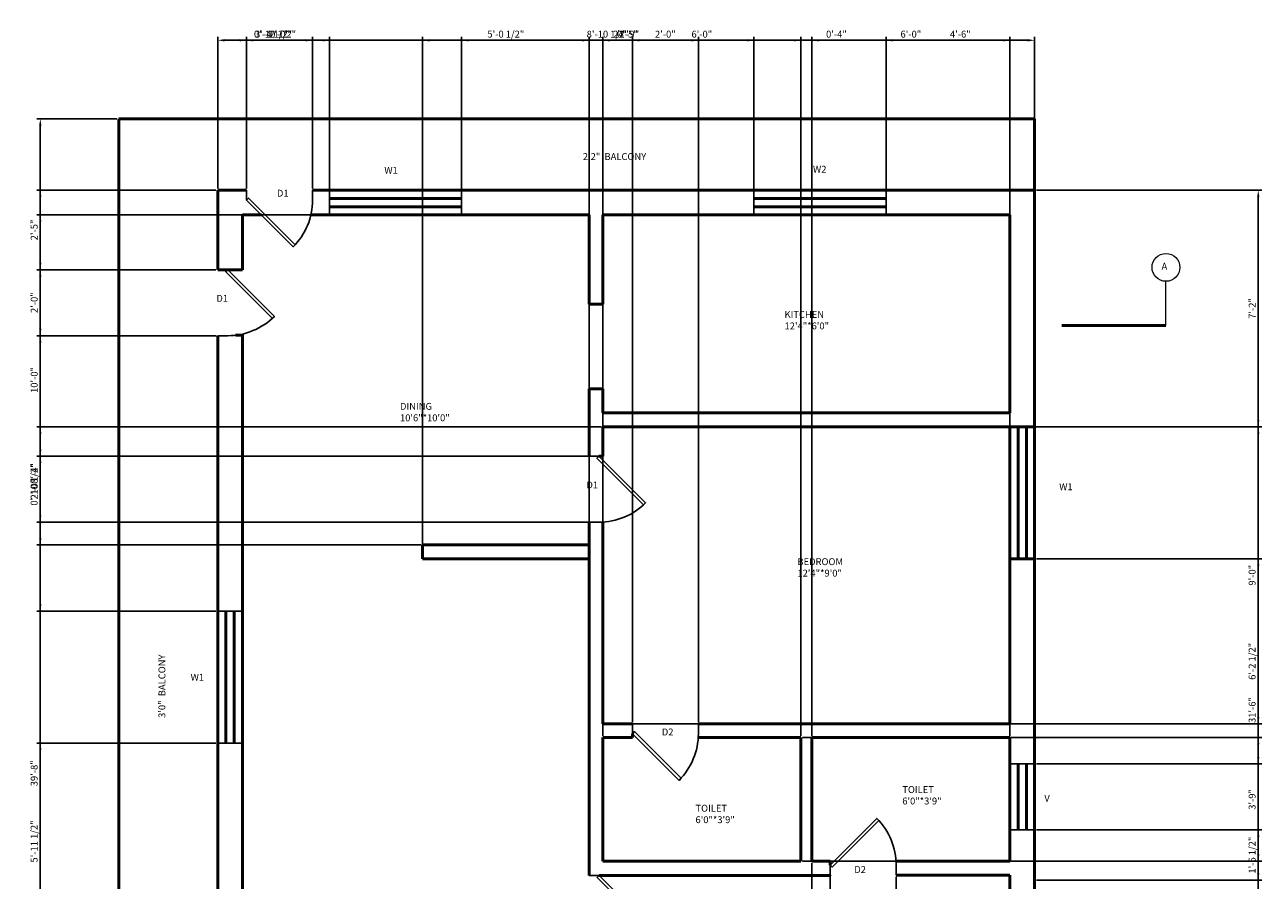
# Model space of a CAD drawing. Units: inches. Extents: x 2020 to 7901, y 1581 to 3943.
# Tile 11 of 17: x 2936 to 3386, y 1963 to 2274. Entities that reach past the tile are written whole.
import ezdxf

# ---------------------------------------------------------------- set-up
doc = ezdxf.new("R2010")
doc.units = ezdxf.units.IN
for name, color, linetype, lineweight in [('A-ANNO-DIMS', 2, 'Continuous', 18), ('A-ANNO-SYMB', 1, 'Continuous', 18), ('A-ANNO-TEXT', 7, 'Continuous', 18), ('A-AREA-IDEN', 3, 'Continuous', 18), ('A-DOOR', 4, 'Continuous', 25), ('A-GLAZ', 4, 'Continuous', 25), ('A-WALL', 7, 'Continuous', 50)]:
    doc.layers.add(name, color=color, linetype=linetype, lineweight=lineweight)
doc.styles.get("Standard").update_dxf_attribs({"font": 'arial.ttf'})
doc.dimstyles.new('ISO-25', dxfattribs={"dimtxt": 2.5, "dimasz": 2.5, "dimexe": 1.25, "dimexo": 0.625, "dimtad": 1, "dimdec": 1, "dimlunit": 3, "dimtxsty": 'Standard', "dimcen": 2.5, "dimadec": 0, "dimazin": 0, "dimtfac": 1, "dimtdec": 1, "dimtmove": 0, "dimatfit": 3, "dimfxl": 1, "dimarcsym": 0})

# ---------------------------------------------------------------- blocks, each defined once
blk = doc.blocks.new('*U10')
for p, q in [((0, 0), (0, -6)), ((40, 0), (40, -6))]:
    blk.add_line(p, q)
blk.add_lwpolyline([(0, 0), (28.28, 28.28), (29.52, 27.05), (1.24, -1.24)], close=True)
blk.add_arc((0, 0), 40, 0, 45)
blk = doc.blocks.new('WIN-1200')
for p, q in [((0, 9), (48, 9)), ((0, 0), (0, 9)), ((48, 9), (48, 0)), ((48, 0), (0, 0))]:
    blk.add_line(p, q)
blk = doc.blocks.new('VENT-600')
for p, q in [((0, 24), (9, 24)), ((0, 24), (0, 0)), ((9, 0), (9, 24)), ((0, 0), (9, 0))]:
    blk.add_line(p, q)
blk = doc.blocks.new('*D44')
at = {"layer": 'A-ANNO-DIMS', "color": 0, "lineweight": -2, "transparency": 16777216}
for p, q in [((3006.32, 2214.96), (3006.32, 2270.09)), ((3046.95, 2214.96), (3046.95, 2270.09)), ((3008.82, 2268.84), (3044.45, 2268.84))]:
    blk.add_line(p, q, dxfattribs=at)
at = {"layer": 'A-ANNO-DIMS', "color": 0, "transparency": 16777216}
for points in [[(3008.82, 2269.26), (3008.82, 2268.42), (3006.32, 2268.84)], [(3044.45, 2269.26), (3044.45, 2268.42), (3046.95, 2268.84)]]:
    blk.add_solid(points, dxfattribs=at)
at = {"layer": 'DEFPOINTS', "color": 0, "transparency": 16777216}
for p in [(3046.95, 2268.84), (3006.32, 2214.34), (3046.95, 2214.34)]:
    blk.add_point(p, dxfattribs=at)
at = {"layer": 'A-ANNO-DIMS', "color": 0, "transparency": 16777216, "insert": (3026.63, 2270.76), "char_height": 2.5, "attachment_point": 5}
blk.add_mtext('3\'-4 1/2"', dxfattribs=at)
blk = doc.blocks.new('*D45')
at = {"layer": 'A-ANNO-DIMS', "color": 0, "lineweight": -2, "transparency": 16777216}
for p, q in [((3094.95, 2214.96), (3094.95, 2270.09)), ((3201.28, 2214.96), (3201.28, 2270.09)), ((3097.45, 2268.84), (3198.78, 2268.84))]:
    blk.add_line(p, q, dxfattribs=at)
at = {"layer": 'A-ANNO-DIMS', "color": 0, "transparency": 16777216}
for points in [[(3097.45, 2269.26), (3097.45, 2268.42), (3094.95, 2268.84)], [(3198.78, 2269.26), (3198.78, 2268.42), (3201.28, 2268.84)]]:
    blk.add_solid(points, dxfattribs=at)
at = {"layer": 'DEFPOINTS', "color": 0, "transparency": 16777216}
for p in [(3201.28, 2268.84), (3094.95, 2214.34), (3201.28, 2214.34)]:
    blk.add_point(p, dxfattribs=at)
at = {"layer": 'A-ANNO-DIMS', "color": 0, "transparency": 16777216, "insert": (3148.11, 2270.76), "char_height": 2.5, "attachment_point": 5}
blk.add_mtext('8\'-10 1/2"', dxfattribs=at)
blk = doc.blocks.new('*D46')
at = {"layer": 'A-ANNO-DIMS', "color": 0, "lineweight": -2, "transparency": 16777216}
for p, q in [((3249.28, 2214.96), (3249.28, 2270.09)), ((3303.32, 2214.96), (3303.32, 2270.09)), ((3251.78, 2268.84), (3300.82, 2268.84))]:
    blk.add_line(p, q, dxfattribs=at)
at = {"layer": 'A-ANNO-DIMS', "color": 0, "transparency": 16777216}
for points in [[(3251.78, 2269.26), (3251.78, 2268.42), (3249.28, 2268.84)], [(3300.82, 2269.26), (3300.82, 2268.42), (3303.32, 2268.84)]]:
    blk.add_solid(points, dxfattribs=at)
at = {"layer": 'DEFPOINTS', "color": 0, "transparency": 16777216}
for p in [(3303.32, 2268.84), (3249.28, 2214.34), (3303.32, 2214.34)]:
    blk.add_point(p, dxfattribs=at)
at = {"layer": 'A-ANNO-DIMS', "color": 0, "transparency": 16777216, "insert": (3276.3, 2270.74), "char_height": 2.5, "attachment_point": 5}
blk.add_mtext('4\'-6"', dxfattribs=at)
blk = doc.blocks.new('*D47')
at = {"layer": 'A-ANNO-DIMS', "color": 0, "lineweight": -2, "transparency": 16777216}
for p, q in [((3303.94, 2214.34), (3385.87, 2214.34)), ((3384.62, 2211.84), (3384.62, 2130.84)), ((3303.94, 2128.34), (3385.87, 2128.34))]:
    blk.add_line(p, q, dxfattribs=at)
at = {"layer": 'A-ANNO-DIMS', "color": 0, "transparency": 16777216}
for points in [[(3384.2, 2211.84), (3385.03, 2211.84), (3384.62, 2214.34)], [(3384.2, 2130.84), (3385.03, 2130.84), (3384.62, 2128.34)]]:
    blk.add_solid(points, dxfattribs=at)
at = {"layer": 'DEFPOINTS', "color": 0, "transparency": 16777216}
for p in [(3303.32, 2214.34), (3303.32, 2128.34), (3384.62, 2128.34)]:
    blk.add_point(p, dxfattribs=at)
at = {"layer": 'A-ANNO-DIMS', "color": 0, "transparency": 16777216, "insert": (3382.74, 2171.34), "char_height": 2.5, "attachment_point": 5, "rotation": 90}
blk.add_mtext('7\'-2"', dxfattribs=at)
blk = doc.blocks.new('*D48')
at = {"layer": 'A-ANNO-DIMS', "color": 0, "lineweight": -2, "transparency": 16777216}
for p, q in [((3303.94, 2080.34), (3385.87, 2080.34)), ((3384.62, 2077.84), (3384.62, 2008.22)), ((3303.94, 2005.72), (3385.87, 2005.72))]:
    blk.add_line(p, q, dxfattribs=at)
at = {"layer": 'A-ANNO-DIMS', "color": 0, "transparency": 16777216}
for points in [[(3384.2, 2077.84), (3385.03, 2077.84), (3384.62, 2080.34)], [(3384.2, 2008.22), (3385.03, 2008.22), (3384.62, 2005.72)]]:
    blk.add_solid(points, dxfattribs=at)
at = {"layer": 'DEFPOINTS', "color": 0, "transparency": 16777216}
for p in [(3303.32, 2080.34), (3303.32, 2005.72), (3384.62, 2005.72)]:
    blk.add_point(p, dxfattribs=at)
at = {"layer": 'A-ANNO-DIMS', "color": 0, "transparency": 16777216, "insert": (3382.7, 2043.03), "char_height": 2.5, "attachment_point": 5, "rotation": 90}
blk.add_mtext('6\'-2 1/2"', dxfattribs=at)
blk = doc.blocks.new('*D49')
at = {"layer": 'A-ANNO-DIMS', "color": 0, "lineweight": -2, "transparency": 16777216}
for p, q in [((3303.94, 1981.72), (3385.87, 1981.72)), ((3384.62, 1979.22), (3384.62, 1965.95)), ((3303.94, 1963.45), (3385.87, 1963.45))]:
    blk.add_line(p, q, dxfattribs=at)
at = {"layer": 'A-ANNO-DIMS', "color": 0, "transparency": 16777216}
for points in [[(3384.2, 1979.22), (3385.03, 1979.22), (3384.62, 1981.72)], [(3384.2, 1965.95), (3385.03, 1965.95), (3384.62, 1963.45)]]:
    blk.add_solid(points, dxfattribs=at)
at = {"layer": 'DEFPOINTS', "color": 0, "transparency": 16777216}
for p in [(3303.32, 1981.72), (3303.32, 1963.45), (3384.62, 1963.45)]:
    blk.add_point(p, dxfattribs=at)
at = {"layer": 'A-ANNO-DIMS', "color": 0, "transparency": 16777216, "insert": (3382.7, 1972.58), "char_height": 2.5, "attachment_point": 5, "rotation": 90}
blk.add_mtext('1\'-6 1/2"', dxfattribs=at)
blk = doc.blocks.new('*D55')
at = {"layer": 'A-ANNO-DIMS', "color": 0, "lineweight": -2, "transparency": 16777216}
for p, q in [((2969.69, 2240.34), (2940.57, 2240.34)), ((2941.82, 2237.84), (2941.82, 1766.84)), ((2969.69, 1764.34), (2940.57, 1764.34))]:
    blk.add_line(p, q, dxfattribs=at)
at = {"layer": 'A-ANNO-DIMS', "color": 0, "transparency": 16777216}
for points in [[(2941.4, 2237.84), (2942.23, 2237.84), (2941.82, 2240.34)], [(2941.4, 1766.84), (2942.23, 1766.84), (2941.82, 1764.34)]]:
    blk.add_solid(points, dxfattribs=at)
at = {"layer": 'DEFPOINTS', "color": 0, "transparency": 16777216}
for p in [(2970.32, 2240.34), (2941.82, 1764.34), (2970.32, 1764.34)]:
    blk.add_point(p, dxfattribs=at)
at = {"layer": 'A-ANNO-DIMS', "color": 0, "transparency": 16777216, "insert": (2939.91, 2002.34), "char_height": 2.5, "attachment_point": 5, "rotation": 90}
blk.add_mtext('39\'-8"', dxfattribs=at)
blk = doc.blocks.new('*D58')
at = {"layer": 'A-ANNO-DIMS', "color": 0, "lineweight": -2, "transparency": 16777216}
for p, q in [((3141.33, 2094.26), (3141.33, 2270.09)), ((3146.32, 2094.3), (3146.32, 2270.09)), ((3138.83, 2268.84), (3136.33, 2268.84)), ((3141.33, 2268.84), (3146.32, 2268.84)), ((3148.82, 2268.84), (3159.21, 2268.84))]:
    blk.add_line(p, q, dxfattribs=at)
at = {"layer": 'A-ANNO-DIMS', "color": 0, "transparency": 16777216}
for points in [[(3138.83, 2269.26), (3138.83, 2268.42), (3141.33, 2268.84)], [(3148.82, 2269.26), (3148.82, 2268.42), (3146.32, 2268.84)]]:
    blk.add_solid(points, dxfattribs=at)
at = {"layer": 'DEFPOINTS', "color": 0, "transparency": 16777216}
for p in [(3146.32, 2268.84), (3141.33, 2093.64), (3146.32, 2093.68)]:
    blk.add_point(p, dxfattribs=at)
at = {"layer": 'A-ANNO-DIMS', "color": 0, "transparency": 16777216, "insert": (3155.26, 2270.74), "char_height": 2.5, "attachment_point": 5}
blk.add_mtext('0\'-5"', dxfattribs=at)
blk = doc.blocks.new('*D59')
at = {"layer": 'A-ANNO-DIMS', "color": 0, "lineweight": -2, "transparency": 16777216}
for p, q in [((3157.06, 2020.96), (3157.06, 2270.09)), ((3181.06, 2020.96), (3181.06, 2270.09)), ((3159.56, 2268.84), (3178.56, 2268.84))]:
    blk.add_line(p, q, dxfattribs=at)
at = {"layer": 'A-ANNO-DIMS', "color": 0, "transparency": 16777216}
for points in [[(3159.56, 2269.26), (3159.56, 2268.42), (3157.06, 2268.84)], [(3178.56, 2269.26), (3178.56, 2268.42), (3181.06, 2268.84)]]:
    blk.add_solid(points, dxfattribs=at)
at = {"layer": 'DEFPOINTS', "color": 0, "transparency": 16777216}
for p in [(3181.06, 2268.84), (3157.06, 2020.34), (3181.06, 2020.34)]:
    blk.add_point(p, dxfattribs=at)
at = {"layer": 'A-ANNO-DIMS', "color": 0, "transparency": 16777216, "insert": (3169.06, 2270.74), "char_height": 2.5, "attachment_point": 5}
blk.add_mtext('2\'-0"', dxfattribs=at)
blk = doc.blocks.new('*D122')
at = {"layer": 'A-ANNO-DIMS', "color": 0, "lineweight": -2, "transparency": 16777216}
for p, q in [((3006.32, 2214.96), (3006.32, 2270.09)), ((3303.32, 2214.96), (3303.32, 2270.09)), ((3008.82, 2268.84), (3300.82, 2268.84))]:
    blk.add_line(p, q, dxfattribs=at)
at = {"layer": 'A-ANNO-DIMS', "color": 0, "transparency": 16777216}
for points in [[(3008.82, 2269.26), (3008.82, 2268.42), (3006.32, 2268.84)], [(3300.82, 2269.26), (3300.82, 2268.42), (3303.32, 2268.84)]]:
    blk.add_solid(points, dxfattribs=at)
at = {"layer": 'DEFPOINTS', "color": 0, "transparency": 16777216}
for p in [(3303.32, 2268.84), (3006.32, 2214.34), (3303.32, 2214.34)]:
    blk.add_point(p, dxfattribs=at)
at = {"layer": 'A-ANNO-DIMS', "color": 0, "transparency": 16777216, "insert": (3154.82, 2270.74), "char_height": 2.5, "attachment_point": 5}
blk.add_mtext('24\'-9"', dxfattribs=at)
blk = doc.blocks.new('*D123')
at = {"layer": 'A-ANNO-DIMS', "color": 0, "lineweight": -2, "transparency": 16777216}
for p, q in [((3303.94, 2214.34), (3385.87, 2214.34)), ((3384.62, 2211.84), (3384.62, 1838.84)), ((3303.94, 1836.34), (3385.87, 1836.34))]:
    blk.add_line(p, q, dxfattribs=at)
at = {"layer": 'A-ANNO-DIMS', "color": 0, "transparency": 16777216}
for points in [[(3384.2, 2211.84), (3385.03, 2211.84), (3384.62, 2214.34)], [(3384.2, 1838.84), (3385.03, 1838.84), (3384.62, 1836.34)]]:
    blk.add_solid(points, dxfattribs=at)
at = {"layer": 'DEFPOINTS', "color": 0, "transparency": 16777216}
for p in [(3303.32, 2214.34), (3303.32, 1836.34), (3384.62, 1836.34)]:
    blk.add_point(p, dxfattribs=at)
at = {"layer": 'A-ANNO-DIMS', "color": 0, "transparency": 16777216, "insert": (3382.71, 2025.34), "char_height": 2.5, "attachment_point": 5, "rotation": 90}
blk.add_mtext('31\'-6"', dxfattribs=at)
blk = doc.blocks.new('*D124')
at = {"layer": 'A-ANNO-DIMS', "color": 0, "lineweight": -2, "transparency": 16777216}
for p, q in [((3006.32, 2214.96), (3006.32, 2270.09)), ((3016.81, 2214.96), (3016.81, 2270.09)), ((3008.82, 2268.84), (3014.31, 2268.84)), ((3016.81, 2268.84), (3034.97, 2268.84))]:
    blk.add_line(p, q, dxfattribs=at)
at = {"layer": 'A-ANNO-DIMS', "color": 0, "transparency": 16777216}
for points in [[(3008.82, 2269.26), (3008.82, 2268.42), (3006.32, 2268.84)], [(3014.31, 2269.26), (3014.31, 2268.42), (3016.81, 2268.84)]]:
    blk.add_solid(points, dxfattribs=at)
at = {"layer": 'DEFPOINTS', "color": 0, "transparency": 16777216}
for p in [(3016.81, 2268.84), (3006.32, 2214.34), (3016.81, 2214.34)]:
    blk.add_point(p, dxfattribs=at)
at = {"layer": 'A-ANNO-DIMS', "color": 0, "transparency": 16777216, "insert": (3027.14, 2270.76), "char_height": 2.5, "attachment_point": 5}
blk.add_mtext('0\'-10 1/2"', dxfattribs=at)
blk = doc.blocks.new('*D125')
at = {"layer": 'A-ANNO-DIMS', "color": 0, "lineweight": -2, "transparency": 16777216}
for p, q in [((3016.81, 2214.96), (3016.81, 2270.09)), ((3040.81, 2214.96), (3040.81, 2270.09)), ((3019.31, 2268.84), (3038.31, 2268.84))]:
    blk.add_line(p, q, dxfattribs=at)
at = {"layer": 'A-ANNO-DIMS', "color": 0, "transparency": 16777216}
for points in [[(3019.31, 2269.26), (3019.31, 2268.42), (3016.81, 2268.84)], [(3038.31, 2269.26), (3038.31, 2268.42), (3040.81, 2268.84)]]:
    blk.add_solid(points, dxfattribs=at)
at = {"layer": 'DEFPOINTS', "color": 0, "transparency": 16777216}
for p in [(3040.81, 2268.84), (3016.81, 2214.34), (3040.81, 2214.34)]:
    blk.add_point(p, dxfattribs=at)
at = {"layer": 'A-ANNO-DIMS', "color": 0, "transparency": 16777216, "insert": (3028.81, 2270.74), "char_height": 2.5, "attachment_point": 5}
blk.add_mtext('2\'-0"', dxfattribs=at)
blk = doc.blocks.new('*D126')
at = {"layer": 'A-ANNO-DIMS', "color": 0, "lineweight": -2, "transparency": 16777216}
for p, q in [((3146.94, 2128.34), (3385.87, 2128.34)), ((3384.62, 2125.84), (3384.62, 2022.84)), ((3146.94, 2020.34), (3385.87, 2020.34))]:
    blk.add_line(p, q, dxfattribs=at)
at = {"layer": 'A-ANNO-DIMS', "color": 0, "transparency": 16777216}
for points in [[(3384.2, 2125.84), (3385.03, 2125.84), (3384.62, 2128.34)], [(3384.2, 2022.84), (3385.03, 2022.84), (3384.62, 2020.34)]]:
    blk.add_solid(points, dxfattribs=at)
at = {"layer": 'DEFPOINTS', "color": 0, "transparency": 16777216}
for p in [(3146.32, 2128.34), (3146.32, 2020.34), (3384.62, 2020.34)]:
    blk.add_point(p, dxfattribs=at)
at = {"layer": 'A-ANNO-DIMS', "color": 0, "transparency": 16777216, "insert": (3382.71, 2074.34), "char_height": 2.5, "attachment_point": 5, "rotation": 90}
blk.add_mtext('9\'-0"', dxfattribs=at)
blk = doc.blocks.new('*D127')
at = {"layer": 'A-ANNO-DIMS', "color": 0, "lineweight": -2, "transparency": 16777216}
for p, q in [((3218.94, 2015.34), (3385.87, 2015.34)), ((3384.62, 2012.84), (3384.62, 1972.84)), ((3218.94, 1970.34), (3385.87, 1970.34))]:
    blk.add_line(p, q, dxfattribs=at)
at = {"layer": 'A-ANNO-DIMS', "color": 0, "transparency": 16777216}
for points in [[(3384.2, 2012.84), (3385.03, 2012.84), (3384.62, 2015.34)], [(3384.2, 1972.84), (3385.03, 1972.84), (3384.62, 1970.34)]]:
    blk.add_solid(points, dxfattribs=at)
at = {"layer": 'DEFPOINTS', "color": 0, "transparency": 16777216}
for p in [(3218.32, 2015.34), (3218.32, 1970.34), (3384.62, 1970.34)]:
    blk.add_point(p, dxfattribs=at)
at = {"layer": 'A-ANNO-DIMS', "color": 0, "transparency": 16777216, "insert": (3382.71, 1992.84), "char_height": 2.5, "attachment_point": 5, "rotation": 90}
blk.add_mtext('3\'-9"', dxfattribs=at)
blk = doc.blocks.new('*D129')
at = {"layer": 'A-ANNO-DIMS', "color": 0, "lineweight": -2, "transparency": 16777216}
for p, q in [((3146.32, 2015.96), (3146.32, 2270.09)), ((3218.32, 2015.96), (3218.32, 2270.09)), ((3148.82, 2268.84), (3215.82, 2268.84))]:
    blk.add_line(p, q, dxfattribs=at)
at = {"layer": 'A-ANNO-DIMS', "color": 0, "transparency": 16777216}
for points in [[(3148.82, 2269.26), (3148.82, 2268.42), (3146.32, 2268.84)], [(3215.82, 2269.26), (3215.82, 2268.42), (3218.32, 2268.84)]]:
    blk.add_solid(points, dxfattribs=at)
at = {"layer": 'DEFPOINTS', "color": 0, "transparency": 16777216}
for p in [(3218.32, 2268.84), (3146.32, 2015.34), (3218.32, 2015.34)]:
    blk.add_point(p, dxfattribs=at)
at = {"layer": 'A-ANNO-DIMS', "color": 0, "transparency": 16777216, "insert": (3182.32, 2270.74), "char_height": 2.5, "attachment_point": 5}
blk.add_mtext('6\'-0"', dxfattribs=at)
blk = doc.blocks.new('*D130')
at = {"layer": 'A-ANNO-DIMS', "color": 0, "lineweight": -2, "transparency": 16777216}
for p, q in [((3218.32, 2015.96), (3218.32, 2270.09)), ((3222.32, 2015.96), (3222.32, 2270.09)), ((3215.82, 2268.84), (3213.32, 2268.84)), ((3218.32, 2268.84), (3222.32, 2268.84)), ((3224.82, 2268.84), (3235.21, 2268.84))]:
    blk.add_line(p, q, dxfattribs=at)
at = {"layer": 'A-ANNO-DIMS', "color": 0, "transparency": 16777216}
for points in [[(3215.82, 2269.26), (3215.82, 2268.42), (3218.32, 2268.84)], [(3224.82, 2269.26), (3224.82, 2268.42), (3222.32, 2268.84)]]:
    blk.add_solid(points, dxfattribs=at)
at = {"layer": 'DEFPOINTS', "color": 0, "transparency": 16777216}
for p in [(3222.32, 2268.84), (3218.32, 2015.34), (3222.32, 2015.34)]:
    blk.add_point(p, dxfattribs=at)
at = {"layer": 'A-ANNO-DIMS', "color": 0, "transparency": 16777216, "insert": (3231.26, 2270.74), "char_height": 2.5, "attachment_point": 5}
blk.add_mtext('0\'-4"', dxfattribs=at)
blk = doc.blocks.new('*D131')
at = {"layer": 'A-ANNO-DIMS', "color": 0, "lineweight": -2, "transparency": 16777216}
for p, q in [((3222.32, 2015.96), (3222.32, 2270.09)), ((3294.32, 2015.96), (3294.32, 2270.09)), ((3224.82, 2268.84), (3291.82, 2268.84))]:
    blk.add_line(p, q, dxfattribs=at)
at = {"layer": 'A-ANNO-DIMS', "color": 0, "transparency": 16777216}
for points in [[(3224.82, 2269.26), (3224.82, 2268.42), (3222.32, 2268.84)], [(3291.82, 2269.26), (3291.82, 2268.42), (3294.32, 2268.84)]]:
    blk.add_solid(points, dxfattribs=at)
at = {"layer": 'DEFPOINTS', "color": 0, "transparency": 16777216}
for p in [(3294.32, 2268.84), (3222.32, 2015.34), (3294.32, 2015.34)]:
    blk.add_point(p, dxfattribs=at)
at = {"layer": 'A-ANNO-DIMS', "color": 0, "transparency": 16777216, "insert": (3258.32, 2270.74), "char_height": 2.5, "attachment_point": 5}
blk.add_mtext('6\'-0"', dxfattribs=at)
blk = doc.blocks.new('*D132')
at = {"layer": 'A-ANNO-DIMS', "color": 0, "lineweight": -2, "transparency": 16777216}
for p, q in [((3094.33, 2205.34), (2940.57, 2205.34)), ((2941.82, 2202.84), (2941.82, 2087.84)), ((3080.19, 2085.34), (2940.57, 2085.34))]:
    blk.add_line(p, q, dxfattribs=at)
at = {"layer": 'A-ANNO-DIMS', "color": 0, "transparency": 16777216}
for points in [[(2941.4, 2202.84), (2942.23, 2202.84), (2941.82, 2205.34)], [(2941.4, 2087.84), (2942.23, 2087.84), (2941.82, 2085.34)]]:
    blk.add_solid(points, dxfattribs=at)
at = {"layer": 'DEFPOINTS', "color": 0, "transparency": 16777216}
for p in [(3094.95, 2205.34), (2941.82, 2085.34), (3080.82, 2085.34)]:
    blk.add_point(p, dxfattribs=at)
at = {"layer": 'A-ANNO-DIMS', "color": 0, "transparency": 16777216, "insert": (2939.92, 2145.34), "char_height": 2.5, "attachment_point": 5, "rotation": 90}
blk.add_mtext('10\'-0"', dxfattribs=at)
blk = doc.blocks.new('*D133')
at = {"layer": 'A-ANNO-DIMS', "color": 0, "lineweight": -2, "transparency": 16777216}
for p, q in [((3080.82, 2080.96), (3080.82, 2270.09)), ((3141.32, 2080.96), (3141.32, 2270.09)), ((3083.32, 2268.84), (3138.82, 2268.84))]:
    blk.add_line(p, q, dxfattribs=at)
at = {"layer": 'A-ANNO-DIMS', "color": 0, "transparency": 16777216}
for points in [[(3083.32, 2269.26), (3083.32, 2268.42), (3080.82, 2268.84)], [(3138.82, 2269.26), (3138.82, 2268.42), (3141.32, 2268.84)]]:
    blk.add_solid(points, dxfattribs=at)
at = {"layer": 'DEFPOINTS', "color": 0, "transparency": 16777216}
for p in [(3141.32, 2268.84), (3080.82, 2080.34), (3141.32, 2080.34)]:
    blk.add_point(p, dxfattribs=at)
at = {"layer": 'A-ANNO-DIMS', "color": 0, "transparency": 16777216, "insert": (3111.07, 2270.76), "char_height": 2.5, "attachment_point": 5}
blk.add_mtext('5\'-0 1/2"', dxfattribs=at)
blk = doc.blocks.new('*D134')
at = {"layer": 'A-ANNO-DIMS', "color": 0, "lineweight": -2, "transparency": 16777216}
for p, q in [((3145.69, 2128.34), (2940.57, 2128.34)), ((2941.82, 2125.84), (2941.82, 2120.14)), ((3145.69, 2117.64), (2940.57, 2117.64)), ((2941.82, 2117.64), (2941.82, 2099.47))]:
    blk.add_line(p, q, dxfattribs=at)
at = {"layer": 'A-ANNO-DIMS', "color": 0, "transparency": 16777216}
for points in [[(2941.4, 2125.84), (2942.23, 2125.84), (2941.82, 2128.34)], [(2941.4, 2120.14), (2942.23, 2120.14), (2941.82, 2117.64)]]:
    blk.add_solid(points, dxfattribs=at)
at = {"layer": 'DEFPOINTS', "color": 0, "transparency": 16777216}
for p in [(3146.32, 2128.34), (2941.82, 2117.64), (3146.32, 2117.64)]:
    blk.add_point(p, dxfattribs=at)
at = {"layer": 'A-ANNO-DIMS', "color": 0, "transparency": 16777216, "insert": (2939.9, 2107.31), "char_height": 2.5, "attachment_point": 5, "rotation": 90}
blk.add_mtext('0\'-10 1/2"', dxfattribs=at)
blk = doc.blocks.new('*D135')
at = {"layer": 'A-ANNO-DIMS', "color": 0, "lineweight": -2, "transparency": 16777216}
for p, q in [((3145.69, 2117.64), (2940.57, 2117.64)), ((2941.82, 2115.14), (2941.82, 2096.18)), ((3145.69, 2093.68), (2940.57, 2093.68))]:
    blk.add_line(p, q, dxfattribs=at)
at = {"layer": 'A-ANNO-DIMS', "color": 0, "transparency": 16777216}
for points in [[(2941.4, 2115.14), (2942.23, 2115.14), (2941.82, 2117.64)], [(2941.4, 2096.18), (2942.23, 2096.18), (2941.82, 2093.68)]]:
    blk.add_solid(points, dxfattribs=at)
at = {"layer": 'DEFPOINTS', "color": 0, "transparency": 16777216}
for p in [(3146.32, 2117.64), (2941.82, 2093.68), (3146.32, 2093.68)]:
    blk.add_point(p, dxfattribs=at)
at = {"layer": 'A-ANNO-DIMS', "color": 0, "transparency": 16777216, "insert": (2939.92, 2105.66), "char_height": 2.5, "attachment_point": 5, "rotation": 90}
blk.add_mtext('2\'-0"', dxfattribs=at)
blk = doc.blocks.new('*D136')
at = {"layer": 'A-ANNO-DIMS', "color": 0, "lineweight": -2, "transparency": 16777216}
for p, q in [((3222.32, 1969.71), (3222.32, 1734.59)), ((3228.97, 1969.71), (3228.97, 1734.59)), ((3224.82, 1735.84), (3226.47, 1735.84)), ((3228.97, 1735.84), (3245.19, 1735.84))]:
    blk.add_line(p, q, dxfattribs=at)
at = {"layer": 'A-ANNO-DIMS', "color": 0, "transparency": 16777216}
for points in [[(3224.82, 1736.26), (3224.82, 1735.42), (3222.32, 1735.84)], [(3226.47, 1736.26), (3226.47, 1735.42), (3228.97, 1735.84)]]:
    blk.add_solid(points, dxfattribs=at)
at = {"layer": 'DEFPOINTS', "color": 0, "transparency": 16777216}
for p in [(3222.32, 1970.34), (3228.97, 1970.34), (3228.97, 1735.84)]:
    blk.add_point(p, dxfattribs=at)
at = {"layer": 'A-ANNO-DIMS', "color": 0, "transparency": 16777216, "insert": (3238.33, 1737.76), "char_height": 2.5, "attachment_point": 5}
blk.add_mtext('0\'-6 1/2"', dxfattribs=at)
blk = doc.blocks.new('*D137')
at = {"layer": 'A-ANNO-DIMS', "color": 0, "lineweight": -2, "transparency": 16777216}
for p, q in [((3228.97, 1964.72), (3228.97, 1734.59)), ((3252.97, 1964.72), (3252.97, 1734.59)), ((3231.47, 1735.84), (3250.47, 1735.84))]:
    blk.add_line(p, q, dxfattribs=at)
at = {"layer": 'A-ANNO-DIMS', "color": 0, "transparency": 16777216}
for points in [[(3231.47, 1736.26), (3231.47, 1735.42), (3228.97, 1735.84)], [(3250.47, 1736.26), (3250.47, 1735.42), (3252.97, 1735.84)]]:
    blk.add_solid(points, dxfattribs=at)
at = {"layer": 'DEFPOINTS', "color": 0, "transparency": 16777216}
for p in [(3228.97, 1965.35), (3252.97, 1965.35), (3252.97, 1735.84)]:
    blk.add_point(p, dxfattribs=at)
at = {"layer": 'A-ANNO-DIMS', "color": 0, "transparency": 16777216, "insert": (3240.97, 1737.74), "char_height": 2.5, "attachment_point": 5}
blk.add_mtext('2\'-0"', dxfattribs=at)
blk = doc.blocks.new('*D140')
at = {"layer": 'A-ANNO-DIMS', "color": 0, "lineweight": -2, "transparency": 16777216}
for p, q in [((3005.69, 2214.34), (2940.57, 2214.34)), ((2941.82, 2211.84), (2941.82, 2187.94)), ((3005.69, 2185.44), (2940.57, 2185.44))]:
    blk.add_line(p, q, dxfattribs=at)
at = {"layer": 'A-ANNO-DIMS', "color": 0, "transparency": 16777216}
for points in [[(2941.4, 2211.84), (2942.23, 2211.84), (2941.82, 2214.34)], [(2941.4, 2187.94), (2942.23, 2187.94), (2941.82, 2185.44)]]:
    blk.add_solid(points, dxfattribs=at)
at = {"layer": 'DEFPOINTS', "color": 0, "transparency": 16777216}
for p in [(3006.32, 2214.34), (2941.82, 2185.44), (3006.32, 2185.44)]:
    blk.add_point(p, dxfattribs=at)
at = {"layer": 'A-ANNO-DIMS', "color": 0, "transparency": 16777216, "insert": (2939.92, 2199.89), "char_height": 2.5, "attachment_point": 5, "rotation": 90}
blk.add_mtext('2\'-5"', dxfattribs=at)
blk = doc.blocks.new('*D141')
at = {"layer": 'A-ANNO-DIMS', "color": 0, "lineweight": -2, "transparency": 16777216}
for p, q in [((3005.69, 2185.44), (2940.57, 2185.44)), ((2941.82, 2182.94), (2941.82, 2163.94)), ((3005.73, 2161.44), (2940.57, 2161.44))]:
    blk.add_line(p, q, dxfattribs=at)
at = {"layer": 'A-ANNO-DIMS', "color": 0, "transparency": 16777216}
for points in [[(2941.4, 2182.94), (2942.23, 2182.94), (2941.82, 2185.44)], [(2941.4, 2163.94), (2942.23, 2163.94), (2941.82, 2161.44)]]:
    blk.add_solid(points, dxfattribs=at)
at = {"layer": 'DEFPOINTS', "color": 0, "transparency": 16777216}
for p in [(3006.32, 2185.44), (2941.82, 2161.44), (3006.36, 2161.44)]:
    blk.add_point(p, dxfattribs=at)
at = {"layer": 'A-ANNO-DIMS', "color": 0, "transparency": 16777216, "insert": (2939.92, 2173.44), "char_height": 2.5, "attachment_point": 5, "rotation": 90}
blk.add_mtext('2\'-0"', dxfattribs=at)
blk = doc.blocks.new('*D142')
at = {"layer": 'A-ANNO-DIMS', "color": 0, "lineweight": -2, "transparency": 16777216}
for p, q in [((3005.73, 2161.44), (2940.57, 2161.44)), ((2941.82, 2158.94), (2941.82, 2063.8)), ((3005.69, 2061.3), (2940.57, 2061.3))]:
    blk.add_line(p, q, dxfattribs=at)
at = {"layer": 'A-ANNO-DIMS', "color": 0, "transparency": 16777216}
for points in [[(2941.4, 2158.94), (2942.23, 2158.94), (2941.82, 2161.44)], [(2941.4, 2063.8), (2942.23, 2063.8), (2941.82, 2061.3)]]:
    blk.add_solid(points, dxfattribs=at)
at = {"layer": 'DEFPOINTS', "color": 0, "transparency": 16777216}
for p in [(3006.36, 2161.44), (2941.82, 2061.3), (3006.32, 2061.3)]:
    blk.add_point(p, dxfattribs=at)
at = {"layer": 'A-ANNO-DIMS', "color": 0, "transparency": 16777216, "insert": (2939.92, 2111.37), "char_height": 2.5, "attachment_point": 5, "rotation": 90}
blk.add_mtext('8\'-4"', dxfattribs=at)
blk = doc.blocks.new('*D143')
at = {"layer": 'A-ANNO-DIMS', "color": 0, "lineweight": -2, "transparency": 16777216}
for p, q in [((3005.69, 2013.3), (2940.57, 2013.3)), ((2941.82, 2010.8), (2941.82, 1944.29)), ((3005.69, 1941.79), (2940.57, 1941.79))]:
    blk.add_line(p, q, dxfattribs=at)
at = {"layer": 'A-ANNO-DIMS', "color": 0, "transparency": 16777216}
for points in [[(2941.4, 2010.8), (2942.23, 2010.8), (2941.82, 2013.3)], [(2941.4, 1944.29), (2942.23, 1944.29), (2941.82, 1941.79)]]:
    blk.add_solid(points, dxfattribs=at)
at = {"layer": 'DEFPOINTS', "color": 0, "transparency": 16777216}
for p in [(3006.32, 2013.3), (2941.82, 1941.79), (3006.32, 1941.79)]:
    blk.add_point(p, dxfattribs=at)
at = {"layer": 'A-ANNO-DIMS', "color": 0, "transparency": 16777216, "insert": (2939.9, 1977.54), "char_height": 2.5, "attachment_point": 5, "rotation": 90}
blk.add_mtext('5\'-11 1/2"', dxfattribs=at)

msp = doc.modelspace()

# ---------------------------------------------------------------- linework, layer by layer
at = {"layer": 'A-ANNO-SYMB'}
msp.add_line((3351.06, 2165.1), (3351.06, 2181.22), dxfattribs=at)
msp.add_circle((3351.06, 2186.28), 5.06, dxfattribs=at)
at = {"layer": 'A-WALL'}
for p, q in [((2970.32, 2240.34), (3303.32, 2240.34)), ((2970.32, 2214.34), (2970.32, 2240.34)), ((3303.32, 2240.34), (3303.32, 1764.34)), ((2970.32, 2214.34), (2970.32, 1836.34)), ((3006.32, 2214.34), (3016.81, 2214.34)), ((3006.32, 2214.34), (3006.32, 2185.44)), ((3040.81, 2214.34), (3303.32, 2214.34)), ((3046.95, 2211.34), (3094.95, 2211.34)), ((3201.28, 2211.34), (3249.28, 2211.34)), ((3094.95, 2208.34), (3046.95, 2208.34)), ((3249.28, 2208.34), (3201.28, 2208.34)), ((3015.32, 2205.34), (3015.32, 2185.44)), ((3015.32, 2205.34), (3022.21, 2205.34)), ((3040.19, 2205.34), (3141.32, 2205.34)), ((3141.32, 2172.96), (3141.32, 2205.34)), ((3146.32, 2205.34), (3146.32, 2172.96)), ((3146.32, 2205.34), (3294.32, 2205.34)), ((3294.32, 2205.34), (3294.32, 2133.34)), ((3006.36, 2185.44), (3015.32, 2185.44)), ((3141.32, 2172.96), (3146.32, 2172.96)), ((3006.36, 2161.44), (3006.36, 1836.34)), ((3012.79, 2161.6), (3015.32, 2161.67)), ((3015.32, 2162.04), (3015.32, 1845.34)), ((3313.16, 2165.1), (3351.06, 2165.1)), ((3141.32, 2133.34), (3141.32, 2142.13)), ((3141.32, 2142.13), (3146.32, 2142.13)), ((3146.32, 2142.13), (3146.32, 2133.34)), ((3141.32, 2133.34), (3141.33, 2117.64)), ((3146.32, 2133.34), (3294.32, 2133.34)), ((3146.32, 2128.34), (3303.32, 2128.34)), ((3146.32, 2128.34), (3146.32, 2117.64)), ((3294.32, 2080.34), (3294.32, 2128.34)), ((3294.32, 2128.34), (3303.32, 2128.34)), ((3294.32, 2128.34), (3294.32, 2020.34)), ((3297.32, 2080.34), (3297.32, 2128.34)), ((3300.32, 2128.34), (3300.32, 2080.34)), ((3303.32, 2128.34), (3303.32, 2080.34)), ((3144.93, 2117.64), (3146.32, 2117.64)), ((3141.33, 2093.64), (3141.33, 1965.19)), ((3146.32, 2093.68), (3146.32, 2020.34)), ((3006.32, 2085.34), (3006.36, 2085.34)), ((3080.82, 2085.34), (3141.32, 2085.34)), ((3080.82, 2080.34), (3080.82, 2085.34)), ((3006.32, 2080.34), (3006.36, 2080.34)), ((3080.82, 2080.34), (3141.32, 2080.34)), ((3303.32, 2080.34), (3294.32, 2080.34)), ((3009.32, 2013.3), (3009.32, 2061.3)), ((3012.32, 2061.3), (3012.32, 2013.3)), ((3141.32, 2020.34), (3141.33, 2020.34)), ((3146.32, 2020.34), (3157.06, 2020.34)), ((3181.06, 2020.34), (3294.32, 2020.34)), ((3141.32, 2015.34), (3141.33, 2015.34)), ((3146.32, 2015.34), (3157.06, 2015.34)), ((3146.32, 2015.34), (3146.32, 1970.34)), ((3157.06, 2016.74), (3157.06, 2015.34)), ((3181.02, 2015.34), (3218.32, 2015.34)), ((3218.32, 2015.34), (3218.32, 1970.34)), ((3222.32, 2015.34), (3222.32, 1970.34)), ((3222.32, 2015.34), (3294.32, 2015.34)), ((3294.32, 2015.34), (3294.32, 1970.34)), ((3297.32, 2005.72), (3297.32, 1981.72)), ((3300.32, 1981.72), (3300.32, 2005.72)), ((3141.32, 1970.34), (3141.33, 1970.34)), ((3146.32, 1970.34), (3218.32, 1970.34)), ((3222.32, 1970.34), (3228.97, 1970.34)), ((3228.97, 1968.95), (3228.97, 1970.34)), ((3252.93, 1970.34), (3294.32, 1970.34)), ((3141.32, 1965.34), (3141.33, 1965.34)), ((3144.99, 1965.19), (3228.97, 1965.19)), ((3228.97, 1965.35), (3228.97, 1965.19)), ((3252.97, 1965.35), (3294.32, 1965.34)), ((3294.32, 1965.34), (3294.32, 1845.34))]:
    msp.add_line(p, q, dxfattribs=at)

# ---------------------------------------------------------------- block references
at = {"layer": 'A-DOOR', "yscale": 0.6, "zscale": 0.6}
for p, xscale, rotation in [((3016.81, 2210.74), -0.6, 180), ((3009.96, 2185.44), 0.6, 270), ((3144.93, 2117.64), 0.6, 270), ((3157.06, 2016.74), -0.6, 180), ((3144.99, 1965.19), 0.6, 270)]:
    msp.add_blockref('*U10', p, dxfattribs=dict(at, xscale=xscale, rotation=rotation))
at = {"layer": 'A-DOOR', "xscale": 0.6, "yscale": 0.6, "zscale": 0.6}
msp.add_blockref('*U10', (3228.97, 1968.95), dxfattribs=at)
at = {"layer": 'A-GLAZ'}
for p in [(3046.95, 2205.34), (3201.28, 2205.34)]:
    msp.add_blockref('WIN-1200', p, dxfattribs=at)
for name, p, rotation in [('WIN-1200', (3015.32, 2013.3), 89.99999999999991), ('VENT-600', (3303.32, 2005.72), 180)]:
    msp.add_blockref(name, p, dxfattribs=dict(at, rotation=rotation))

# ---------------------------------------------------------------- texts
at = {"layer": 'A-ANNO-SYMB', "insert": (3349.45, 2187.93), "char_height": 2.5, "attachment_point": 1}
msp.add_mtext_dynamic_manual_height_columns('A', width=4.5735, gutter_width=12.5, heights=[0], dxfattribs=at)
at = {"layer": 'A-ANNO-TEXT', "char_height": 2.5, "attachment_point": 1}
for s, width, insert in [('2\'2"  BALCONY', 87.2542, (3139.06, 2227.82)), ('W1', 20.8875, (3066.9, 2222.8)), ('W2', 16.4632, (3222.73, 2223.2)), ('D1', 8.7807, (3027.84, 2214.49)), ('D1', 4.453, (3005.83, 2176.25)), ('D1', 4.781, (3140.37, 2108.42)), ('W1', 20.4288, (3312.26, 2107.77)), ('W1', 9.8645, (2996.47, 2038.49)), ('D2', 9.6246, (3167.78, 2018.6)), ('V', 15.6081, (3306.85, 1994.5)), ('D2', 8.7799, (3237.75, 1968.6))]:
    msp.add_mtext_dynamic_manual_height_columns(s, width=width, gutter_width=12.5, heights=[0], dxfattribs=dict(at, insert=insert))
at = {"layer": 'A-ANNO-TEXT', "insert": (2984.79, 2022.47), "char_height": 2.5, "attachment_point": 1, "rotation": 90}
msp.add_mtext_dynamic_manual_height_columns('3\'0"  BALCONY', width=25.7427, gutter_width=12.5, heights=[0], dxfattribs=at)
at = {"layer": 'A-AREA-IDEN', "char_height": 2.5, "attachment_point": 1}
for s, width, insert in [('KITCHEN\\P12\'4"*6\'0"', 63.7351, (3212.39, 2170.41)), ('DINING\\P10\'6"*10\'0"', 69.2305, (3072.59, 2137)), ('BEDROOM\\P12\'4"*9\'0"', 67.2565, (3217.07, 2080.53)), ('TOILET\\P6\'0"*3\'9"', 28.3675, (3255.2, 1997.67)), ('TOILET\\P6\'0"*3\'9"', 39.3423, (3180.01, 1990.88))]:
    msp.add_mtext_dynamic_manual_height_columns(s, width=width, gutter_width=12.5, heights=[0], dxfattribs=dict(at, insert=insert))

# ---------------------------------------------------------------- dimensions: what is measured, and where the dimension line sits
at = {"layer": 'A-ANNO-DIMS'}
for base, p1, p2, picture, middle in [((3046.95, 2268.84), (3006.32, 2214.34), (3046.95, 2214.34), '*D44', (3026.63, 2270.76)), ((3016.81, 2268.84), (3006.32, 2214.34), (3016.81, 2214.34), '*D124', (3027.14, 2270.76)), ((3141.32, 2268.84), (3080.82, 2080.34), (3141.32, 2080.34), '*D133', (3111.07, 2270.76)), ((3201.28, 2268.84), (3094.95, 2214.34), (3201.28, 2214.34), '*D45', (3148.11, 2270.76)), ((3303.32, 2268.84), (3006.32, 2214.34), (3303.32, 2214.34), '*D122', (3154.82, 2270.74)), ((3040.81, 2268.84), (3016.81, 2214.34), (3040.81, 2214.34), '*D125', (3028.81, 2270.74)), ((3146.32, 2268.84), (3141.33, 2093.64), (3146.32, 2093.68), '*D58', (3155.26, 2270.74)), ((3218.32, 2268.84), (3146.32, 2015.34), (3218.32, 2015.34), '*D129', (3182.32, 2270.74)), ((3181.06, 2268.84), (3157.06, 2020.34), (3181.06, 2020.34), '*D59', (3169.06, 2270.74)), ((3222.32, 2268.84), (3218.32, 2015.34), (3222.32, 2015.34), '*D130', (3231.26, 2270.74)), ((3294.32, 2268.84), (3222.32, 2015.34), (3294.32, 2015.34), '*D131', (3258.32, 2270.74)), ((3303.32, 2268.84), (3249.28, 2214.34), (3303.32, 2214.34), '*D46', (3276.3, 2270.74)), ((3228.9718, 1735.8394), (3222.3165, 1970.3394), (3228.9718, 1970.3394), '*D136', (3238.3323, 1737.7571)), ((3252.97, 1735.84), (3228.97, 1965.35), (3252.97, 1965.35), '*D137', (3240.97, 1737.74))]:
    dim = msp.add_linear_dim(base=base, p1=p1, p2=p2, dimstyle='ISO-25', override={"dimdec": 1, "dimlfac": 1, "dimrnd": 0, "dimzin": 1, "dimdsep": 46, "dimlunit": 4, "dimfrac": 2}, dxfattribs=at)
    dim.commit()
    dim.dimension.update_dxf_attribs({"geometry": picture, "text_midpoint": middle})
for base, p1, p2, picture, middle in [((2941.82, 1764.34), (2970.32, 2240.34), (2970.32, 1764.34), '*D55', (2939.91, 2002.34)), ((2941.82, 2185.44), (3006.32, 2214.34), (3006.32, 2185.44), '*D140', (2939.92, 2199.89)), ((3384.62, 2128.34), (3303.32, 2214.34), (3303.32, 2128.34), '*D47', (3382.74, 2171.34)), ((3384.62, 1836.34), (3303.32, 2214.34), (3303.32, 1836.34), '*D123', (3382.71, 2025.34)), ((2941.82, 2085.34), (3094.95, 2205.34), (3080.82, 2085.34), '*D132', (2939.92, 2145.34)), ((2941.82, 2161.44), (3006.32, 2185.44), (3006.36, 2161.44), '*D141', (2939.92, 2173.44)), ((2941.82, 2061.3), (3006.36, 2161.44), (3006.32, 2061.3), '*D142', (2939.92, 2111.37)), ((2941.82, 2117.64), (3146.32, 2128.34), (3146.32, 2117.64), '*D134', (2939.9, 2107.31)), ((3384.62, 2020.34), (3146.32, 2128.34), (3146.32, 2020.34), '*D126', (3382.71, 2074.34)), ((2941.82, 2093.68), (3146.32, 2117.64), (3146.32, 2093.68), '*D135', (2939.92, 2105.66)), ((3384.62, 2005.72), (3303.32, 2080.34), (3303.32, 2005.72), '*D48', (3382.7, 2043.03)), ((2941.82, 1941.79), (3006.32, 2013.3), (3006.32, 1941.79), '*D143', (2939.9, 1977.54)), ((3384.62, 1970.34), (3218.32, 2015.34), (3218.32, 1970.34), '*D127', (3382.71, 1992.84)), ((3384.62, 1963.45), (3303.32, 1981.72), (3303.32, 1963.45), '*D49', (3382.7, 1972.58))]:
    dim = msp.add_linear_dim(base=base, p1=p1, p2=p2, angle=90, dimstyle='ISO-25', override={"dimdec": 1, "dimlfac": 1, "dimrnd": 0, "dimzin": 1, "dimdsep": 46, "dimlunit": 4, "dimfrac": 2}, dxfattribs=at)
    dim.commit()
    dim.dimension.update_dxf_attribs({"geometry": picture, "text_midpoint": middle})

doc.saveas('drawing.dxf')
